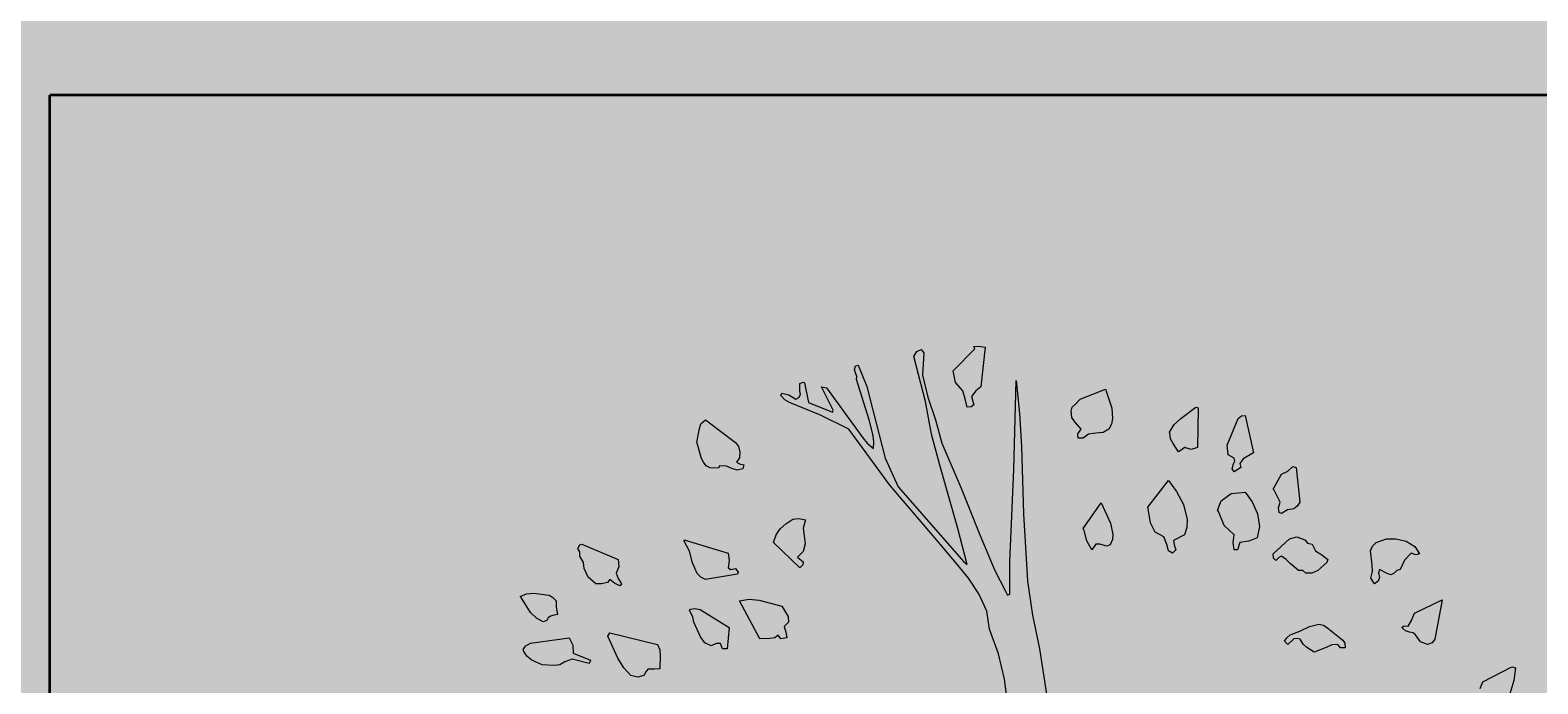
# Model space of a CAD drawing. Units: inches. Extents: x 84 to 1044, y -280 to 906.
# Tile 77 of 105: x 704 to 733, y 500 to 512. Entities that reach past the tile are written whole.
import ezdxf

# ---------------------------------------------------------------- set-up
doc = ezdxf.new("R2010")
doc.units = ezdxf.units.IN
for name, color, linetype, lineweight in [('A-ANNO-DIMS', 2, 'Continuous', 18), ('L-PLNT', 114, 'Continuous', 15), ('WALL', 250, 'Continuous', 35)]:
    doc.layers.add(name, color=color, linetype=linetype, lineweight=lineweight)
doc.layers.add('A-WALL-PATT', color=251, linetype='Continuous', lineweight=9, true_color=0x636466)
doc.layers.add('L-PLNT-PATT', color=9, linetype='Continuous', lineweight=9, true_color=0xafd9aa)
doc.styles.get("Standard").update_dxf_attribs({"font": 'arial.ttf'})
doc.dimstyles.get("Standard").update_dxf_attribs({"dimtxt": 0.18, "dimasz": 0.18, "dimexe": 0.18, "dimexo": 0.0625, "dimgap": 0.09, "dimtad": 0, "dimtih": 1, "dimtoh": 1, "dimdec": 4, "dimzin": 0, "dimdsep": 46, "dimtxsty": 'Standard', "dimcen": 0.09, "dimadec": 0, "dimazin": 0, "dimtfac": 1, "dimtdec": 4, "dimtofl": 0, "dimtmove": 0, "dimatfit": 3, "dimfxl": 1, "dimtolj": 1, "dimtzin": 0, "dimarcsym": 0})

# ---------------------------------------------------------------- blocks, each defined once
blk = doc.blocks.new('A$C37E508DF')
for p, q in [((0.6329, 1.5111), (0.6367, 1.5175)), ((0.6367, 1.5175), (0.6423, 1.5201)), ((0.6423, 1.5201), (0.6453, 1.5158)), ((0.6826, 1.493), (0.7096, 1.5209)), ((0.7083, 1.5239), (0.7152, 1.5244)), ((0.7096, 1.5209), (0.7083, 1.5239)), ((0.7152, 1.5244), (0.7225, 1.5231)), ((0.7225, 1.5231), (0.7174, 1.4729)), ((0.5583, 1.4948), (0.5596, 1.4995)), ((0.5596, 1.4995), (0.563, 1.5003)), ((0.563, 1.5003), (0.5737, 1.4733)), ((0.6475, 1.4545), (0.6329, 1.5111)), ((0.6453, 1.5158), (0.644, 1.4879)), ((0.5596, 1.4905), (0.5583, 1.4948)), ((0.5613, 1.4862), (0.5596, 1.4905)), ((0.5608, 1.4823), (0.5613, 1.4862)), ((0.5767, 1.4317), (0.5608, 1.4823)), ((0.644, 1.4879), (0.6505, 1.46)), ((0.6852, 1.4785), (0.6826, 1.493)), ((0.7589, 1.3691), (0.7615, 1.481)), ((0.7615, 1.481), (0.7658, 1.4395)), ((0.4657, 1.4622), (0.4669, 1.4652)), ((0.4708, 1.4566), (0.4657, 1.4622)), ((0.4669, 1.4652), (0.4755, 1.463)), ((0.4755, 1.463), (0.4845, 1.4575)), ((0.4884, 1.4596), (0.4905, 1.4635)), ((0.4897, 1.4772), (0.4935, 1.4789)), ((0.4897, 1.4678), (0.4897, 1.4772)), ((0.4905, 1.4635), (0.4897, 1.4678)), ((0.4935, 1.4789), (0.4952, 1.478)), ((0.4952, 1.478), (0.5004, 1.4532)), ((0.5313, 1.4437), (0.5167, 1.4729)), ((0.5167, 1.4729), (0.5231, 1.4716)), ((0.5231, 1.4716), (0.5686, 1.409)), ((0.5737, 1.4733), (0.5814, 1.4437)), ((0.6946, 1.4682), (0.6852, 1.4785)), ((0.6976, 1.4579), (0.6946, 1.4682)), ((0.7109, 1.4682), (0.7053, 1.4609)), ((0.7053, 1.4609), (0.7083, 1.4502)), ((0.7174, 1.4729), (0.7109, 1.4682)), ((0.8421, 1.4575), (0.8739, 1.4703)), ((0.8739, 1.4703), (0.882, 1.4463)), ((0.4764, 1.4532), (0.4708, 1.4566)), ((0.5154, 1.4373), (0.4764, 1.4532)), ((0.4845, 1.4575), (0.4884, 1.4596)), ((0.5004, 1.4532), (0.5308, 1.4412)), ((0.5308, 1.4412), (0.5313, 1.4437)), ((0.5814, 1.4437), (0.5969, 1.3833)), ((0.6552, 1.4137), (0.6475, 1.4545)), ((0.6505, 1.46), (0.6603, 1.4317)), ((0.7002, 1.4476), (0.6976, 1.4579)), ((0.7049, 1.448), (0.7002, 1.4476)), ((0.7083, 1.4502), (0.7049, 1.448)), ((0.831, 1.4424), (0.8323, 1.4476)), ((0.8318, 1.4343), (0.831, 1.4424)), ((0.8323, 1.4476), (0.8357, 1.451)), ((0.8357, 1.451), (0.8421, 1.4575)), ((0.882, 1.4463), (0.8829, 1.433)), ((0.9686, 1.4334), (0.9875, 1.4476)), ((0.9875, 1.4476), (0.9905, 1.4467)), ((0.9905, 1.4467), (0.9896, 1.3966)), ((0.3628, 1.4189), (0.3649, 1.4266)), ((0.3649, 1.4266), (0.3709, 1.4317)), ((0.3709, 1.4317), (0.4086, 1.403)), ((0.551, 1.4197), (0.5154, 1.4373)), ((0.5814, 1.4133), (0.5767, 1.4317)), ((0.6603, 1.4317), (0.668, 1.4021)), ((0.7658, 1.4395), (0.7684, 1.3979)), ((0.8353, 1.4292), (0.8318, 1.4343)), ((0.8434, 1.4197), (0.8353, 1.4292)), ((0.8816, 1.4262), (0.8781, 1.4197)), ((0.8829, 1.433), (0.8816, 1.4262)), ((0.9545, 1.4159), (0.9605, 1.4257)), ((0.9605, 1.4257), (0.9686, 1.4334)), ((1.0269, 1.3996), (1.0411, 1.433)), ((1.0411, 1.433), (1.045, 1.4365)), ((1.045, 1.4365), (1.0497, 1.4369)), ((1.0497, 1.4369), (1.0604, 1.3901)), ((0.3598, 1.403), (0.3628, 1.4189)), ((0.6029, 1.3494), (0.551, 1.4197)), ((0.5686, 1.409), (0.5741, 1.4021)), ((0.5827, 1.4043), (0.5814, 1.4133)), ((0.5823, 1.3953), (0.5827, 1.4043)), ((0.6655, 1.3743), (0.6552, 1.4137)), ((0.8391, 1.4141), (0.8434, 1.4197)), ((0.8395, 1.4086), (0.8391, 1.4141)), ((0.846, 1.4086), (0.8395, 1.4086)), ((0.8528, 1.4137), (0.846, 1.4086)), ((0.8619, 1.4146), (0.8528, 1.4137)), ((0.8709, 1.4154), (0.8619, 1.4146)), ((0.8781, 1.4197), (0.8709, 1.4154)), ((0.9549, 1.4146), (0.9545, 1.4159)), ((0.9558, 1.4077), (0.9549, 1.4146)), ((0.9592, 1.4017), (0.9558, 1.4077)), ((0.3602, 1.4021), (0.3598, 1.403)), ((0.364, 1.3888), (0.3602, 1.4021)), ((0.3657, 1.3828), (0.364, 1.3888)), ((0.4086, 1.403), (0.4125, 1.3979)), ((0.4125, 1.3979), (0.4142, 1.391)), ((0.4142, 1.391), (0.4134, 1.3837)), ((0.5741, 1.4021), (0.5823, 1.3953)), ((0.668, 1.4021), (0.6925, 1.3455)), ((0.7684, 1.3979), (0.771, 1.3134)), ((0.966, 1.3914), (0.9592, 1.4017)), ((0.9703, 1.3944), (0.966, 1.3914)), ((0.9733, 1.3966), (0.9703, 1.3944)), ((0.9819, 1.3944), (0.9733, 1.3966)), ((0.9896, 1.3966), (0.9819, 1.3944)), ((1.0282, 1.3876), (1.0269, 1.3996)), ((1.0359, 1.3833), (1.0282, 1.3876)), ((1.0604, 1.3901), (1.0471, 1.3824)), ((0.3683, 1.3781), (0.3657, 1.3828)), ((0.3718, 1.3738), (0.3683, 1.3781)), ((0.3765, 1.3713), (0.3718, 1.3738)), ((0.3872, 1.3708), (0.3765, 1.3713)), ((0.3885, 1.3738), (0.3872, 1.3708)), ((0.3971, 1.3734), (0.3885, 1.3738)), ((0.4039, 1.3704), (0.3971, 1.3734)), ((0.4108, 1.3683), (0.4039, 1.3704)), ((0.4134, 1.3837), (0.4099, 1.3781)), ((0.4099, 1.3781), (0.4134, 1.376)), ((0.4176, 1.37), (0.4108, 1.3683)), ((0.4134, 1.376), (0.4189, 1.3751)), ((0.4189, 1.3751), (0.4176, 1.37)), ((0.5969, 1.3833), (0.6132, 1.3472)), ((0.6882, 1.2949), (0.6655, 1.3743)), ((0.7538, 1.2529), (0.7589, 1.3691)), ((1.0334, 1.37), (1.0351, 1.376)), ((1.0359, 1.3661), (1.0334, 1.37)), ((1.0351, 1.376), (1.0368, 1.3794)), ((1.0368, 1.3794), (1.0359, 1.3833)), ((1.0441, 1.3717), (1.0359, 1.3661)), ((1.0471, 1.3824), (1.0432, 1.3764)), ((1.0432, 1.3764), (1.0441, 1.3717)), ((1.0955, 1.3631), (1.1033, 1.367)), ((1.1033, 1.367), (1.1097, 1.373)), ((1.1097, 1.373), (1.114, 1.3717)), ((1.114, 1.3717), (1.1183, 1.328)), ((0.6595, 1.2829), (0.6029, 1.3494)), ((0.6132, 1.3472), (0.6959, 1.2529)), ((0.9274, 1.3215), (0.9532, 1.3554)), ((0.9532, 1.3554), (0.9635, 1.3413)), ((1.0848, 1.3443), (1.0955, 1.3631)), ((0.6925, 1.3455), (0.7161, 1.2868)), ((0.9635, 1.3413), (0.9721, 1.325)), ((1.0171, 1.3232), (1.0197, 1.3297)), ((1.0197, 1.3297), (1.0321, 1.3387)), ((1.0321, 1.3387), (1.0497, 1.3404)), ((1.0497, 1.3404), (1.0587, 1.3284)), ((1.0587, 1.3284), (1.0651, 1.3134)), ((1.0861, 1.343), (1.0848, 1.3443)), ((1.0938, 1.328), (1.0861, 1.343)), ((1.0917, 1.3207), (1.0938, 1.328)), ((1.1183, 1.328), (1.1153, 1.3228)), ((0.771, 1.3134), (0.7761, 1.2285)), ((0.846, 1.2949), (0.8687, 1.3271)), ((0.8687, 1.3271), (0.8803, 1.3014)), ((0.9279, 1.3194), (0.9274, 1.3215)), ((0.9305, 1.3018), (0.9279, 1.3194)), ((0.9721, 1.325), (0.9768, 1.3061)), ((1.0149, 1.3172), (1.0171, 1.3232)), ((1.0162, 1.3164), (1.0149, 1.3172)), ((1.0231, 1.2988), (1.0162, 1.3164)), ((1.0651, 1.3134), (1.0677, 1.2975)), ((1.0925, 1.3151), (1.0917, 1.3207)), ((1.0955, 1.3138), (1.0925, 1.3151)), ((1.1028, 1.3185), (1.0955, 1.3138)), ((1.111, 1.3194), (1.1028, 1.3185)), ((1.1153, 1.3228), (1.111, 1.3194)), ((0.4597, 1.2868), (0.4648, 1.2945)), ((0.4648, 1.2945), (0.4717, 1.3009)), ((0.4717, 1.3009), (0.4807, 1.3065)), ((0.4807, 1.3065), (0.4884, 1.3074)), ((0.4884, 1.3074), (0.4965, 1.3057)), ((0.4965, 1.3057), (0.4935, 1.2954)), ((0.4935, 1.2954), (0.4948, 1.2855)), ((0.7002, 1.2495), (0.6882, 1.2949)), ((0.8473, 1.2924), (0.846, 1.2949)), ((0.8507, 1.2795), (0.8473, 1.2924)), ((0.8803, 1.3014), (0.8833, 1.2872)), ((0.9365, 1.2902), (0.9305, 1.3018)), ((0.9476, 1.2842), (0.9365, 1.2902)), ((0.9763, 1.2962), (0.9733, 1.2868)), ((0.9768, 1.3061), (0.9763, 1.2962)), ((1.0359, 1.2868), (1.0231, 1.2988)), ((1.0677, 1.2975), (1.0647, 1.2829)), ((0.2101, 1.2696), (0.2127, 1.2744)), ((0.2127, 1.2744), (0.2152, 1.2752)), ((0.2152, 1.2752), (0.2611, 1.2559)), ((0.3439, 1.2804), (0.3992, 1.2636)), ((0.3439, 1.2787), (0.3439, 1.2804)), ((0.3507, 1.2662), (0.3439, 1.2787)), ((0.4562, 1.2774), (0.4597, 1.2868)), ((0.4897, 1.2452), (0.4562, 1.2774)), ((0.4961, 1.2756), (0.4935, 1.2658)), ((0.4948, 1.2855), (0.4961, 1.2756)), ((0.6865, 1.2508), (0.6595, 1.2829)), ((0.7161, 1.2868), (0.7349, 1.2422)), ((0.8567, 1.2679), (0.8507, 1.2795)), ((0.8619, 1.2752), (0.8567, 1.2679)), ((0.867, 1.2752), (0.8619, 1.2752)), ((0.8713, 1.2739), (0.867, 1.2752)), ((0.8756, 1.2726), (0.8713, 1.2739)), ((0.8799, 1.2744), (0.8756, 1.2726)), ((0.8829, 1.2808), (0.8799, 1.2744)), ((0.8833, 1.2872), (0.8829, 1.2808)), ((0.951, 1.2748), (0.9476, 1.2842)), ((0.9532, 1.2666), (0.951, 1.2748)), ((0.9733, 1.2868), (0.9596, 1.2799)), ((0.9596, 1.2799), (0.9605, 1.2744)), ((0.9605, 1.2744), (0.9626, 1.2679)), ((1.0347, 1.2769), (1.0359, 1.2868)), ((1.0359, 1.2679), (1.0347, 1.2769)), ((1.0432, 1.2774), (1.0402, 1.2679)), ((1.0544, 1.2791), (1.0432, 1.2774)), ((1.0647, 1.2829), (1.0544, 1.2791)), ((1.0848, 1.2628), (1.1054, 1.2817)), ((1.1054, 1.2817), (1.1148, 1.2842)), ((1.1148, 1.2842), (1.1247, 1.2804)), ((1.1247, 1.2804), (1.1281, 1.2765)), ((1.1281, 1.2765), (1.1341, 1.2752)), ((1.1341, 1.2752), (1.1384, 1.2666)), ((1.2075, 1.2666), (1.21, 1.2726)), ((1.21, 1.2726), (1.2147, 1.2774)), ((1.2147, 1.2774), (1.2276, 1.2817)), ((1.2276, 1.2817), (1.2392, 1.2817)), ((1.2392, 1.2817), (1.2521, 1.2787)), ((1.2521, 1.2787), (1.2632, 1.2722)), ((1.2632, 1.2722), (1.2692, 1.2628)), ((0.2127, 1.2654), (0.2101, 1.2696)), ((0.2127, 1.2602), (0.2127, 1.2654)), ((0.2174, 1.2521), (0.2127, 1.2602)), ((0.2182, 1.2443), (0.2174, 1.2521)), ((0.2611, 1.2559), (0.262, 1.2465)), ((0.3546, 1.2516), (0.3507, 1.2662)), ((0.3992, 1.2636), (0.4005, 1.2546)), ((0.4005, 1.2546), (0.3992, 1.2452)), ((0.4935, 1.2658), (0.4867, 1.2589)), ((0.4867, 1.2589), (0.4935, 1.2529)), ((0.4935, 1.2529), (0.4931, 1.2491)), ((0.6959, 1.2529), (0.7002, 1.2495)), ((0.7538, 1.2122), (0.7538, 1.2529)), ((0.9583, 1.2636), (0.9532, 1.2666)), ((0.9626, 1.2679), (0.9583, 1.2636)), ((1.0402, 1.2679), (1.0359, 1.2679)), ((1.0852, 1.2576), (1.0848, 1.2628)), ((1.0883, 1.2546), (1.0852, 1.2576)), ((1.0921, 1.2585), (1.0883, 1.2546)), ((1.0955, 1.2602), (1.0921, 1.2585)), ((1.1015, 1.2559), (1.0955, 1.2602)), ((1.1063, 1.2508), (1.1015, 1.2559)), ((1.1384, 1.2666), (1.1461, 1.2619)), ((1.1526, 1.2521), (1.141, 1.2422)), ((1.1461, 1.2619), (1.1539, 1.2559)), ((1.1539, 1.2559), (1.1526, 1.2521)), ((1.2096, 1.2491), (1.2075, 1.2666)), ((1.2503, 1.2551), (1.2448, 1.2431)), ((1.2585, 1.2636), (1.2503, 1.2551)), ((1.2645, 1.2615), (1.2585, 1.2636)), ((1.2692, 1.2628), (1.2645, 1.2615)), ((0.2234, 1.2336), (0.2182, 1.2443)), ((0.2328, 1.2251), (0.2234, 1.2336)), ((0.262, 1.2465), (0.2586, 1.2388)), ((0.2586, 1.2388), (0.2611, 1.2319)), ((0.3602, 1.2383), (0.3546, 1.2516)), ((0.3649, 1.2336), (0.3602, 1.2383)), ((0.3709, 1.2306), (0.3649, 1.2336)), ((0.4112, 1.2375), (0.3709, 1.2306)), ((0.3992, 1.2452), (0.4026, 1.2431)), ((0.4026, 1.2431), (0.4086, 1.2443)), ((0.4086, 1.2443), (0.4121, 1.2401)), ((0.4121, 1.2401), (0.4112, 1.2375)), ((0.4931, 1.2491), (0.4897, 1.2452)), ((0.7015, 1.2323), (0.6865, 1.2508)), ((0.7349, 1.2422), (0.7482, 1.216)), ((1.117, 1.2422), (1.1063, 1.2508)), ((1.1221, 1.2418), (1.117, 1.2422)), ((1.126, 1.2388), (1.1221, 1.2418)), ((1.1337, 1.2388), (1.126, 1.2388)), ((1.141, 1.2422), (1.1337, 1.2388)), ((1.2079, 1.2323), (1.21, 1.2409)), ((1.21, 1.2409), (1.2096, 1.2491)), ((1.2186, 1.2332), (1.2169, 1.2285)), ((1.2186, 1.2431), (1.2173, 1.2392)), ((1.2173, 1.2392), (1.2186, 1.2332)), ((1.2285, 1.2383), (1.2186, 1.2431)), ((1.2328, 1.2366), (1.2285, 1.2383)), ((1.2371, 1.2388), (1.2328, 1.2366)), ((1.2405, 1.2418), (1.2371, 1.2388)), ((1.2448, 1.2431), (1.2405, 1.2418)), ((0.2401, 1.2251), (0.2328, 1.2251)), ((0.2474, 1.2268), (0.2401, 1.2251)), ((0.2504, 1.2306), (0.2474, 1.2268)), ((0.2568, 1.2255), (0.2504, 1.2306)), ((0.2633, 1.2229), (0.2568, 1.2255)), ((0.2611, 1.2319), (0.265, 1.2251)), ((0.265, 1.2251), (0.2633, 1.2229)), ((0.7148, 1.2126), (0.7015, 1.2323)), ((0.7482, 1.216), (0.7508, 1.2109)), ((0.7761, 1.2285), (0.7821, 1.1856)), ((1.2126, 1.2251), (1.2079, 1.2323)), ((1.2169, 1.2285), (1.2126, 1.2251)), ((0.1376, 1.2092), (0.1458, 1.2126)), ((0.1389, 1.2079), (0.1376, 1.2092)), ((0.1505, 1.189), (0.1389, 1.2079)), ((0.1458, 1.2126), (0.1548, 1.2135)), ((0.1548, 1.2135), (0.1741, 1.2109)), ((0.1741, 1.2109), (0.1784, 1.2083)), ((0.1784, 1.2083), (0.1831, 1.204)), ((0.1831, 1.204), (0.1831, 1.1959)), ((0.1831, 1.1959), (0.1848, 1.1865)), ((0.4134, 1.204), (0.4258, 1.2058)), ((0.4391, 1.156), (0.4134, 1.204)), ((0.4258, 1.2058), (0.4382, 1.2045)), ((0.4382, 1.2045), (0.4669, 1.1972)), ((0.4669, 1.1972), (0.4747, 1.1843)), ((0.7246, 1.1908), (0.7148, 1.2126)), ((0.7508, 1.2109), (0.7538, 1.2122)), ((1.2628, 1.1882), (1.2975, 1.2053)), ((1.2975, 1.2053), (1.2885, 1.1556)), ((0.1582, 1.1822), (0.1505, 1.189)), ((0.1668, 1.1775), (0.1582, 1.1822)), ((0.1711, 1.1792), (0.1668, 1.1775)), ((0.1728, 1.1826), (0.1711, 1.1792)), ((0.1758, 1.1847), (0.1728, 1.1826)), ((0.1788, 1.1852), (0.1758, 1.1847)), ((0.1848, 1.1865), (0.1788, 1.1852)), ((0.3507, 1.1916), (0.352, 1.1933)), ((0.355, 1.1839), (0.3507, 1.1916)), ((0.352, 1.1933), (0.3576, 1.1942)), ((0.3563, 1.177), (0.355, 1.1839)), ((0.3645, 1.1586), (0.3563, 1.177)), ((0.3576, 1.1942), (0.364, 1.1929)), ((0.364, 1.1929), (0.4005, 1.1702)), ((0.4751, 1.177), (0.47, 1.1714)), ((0.4747, 1.1843), (0.4751, 1.177)), ((0.7281, 1.168), (0.7246, 1.1908)), ((0.7821, 1.1856), (0.7911, 1.1436)), ((1.2546, 1.1719), (1.2589, 1.1792)), ((1.2589, 1.1792), (1.2628, 1.1882)), ((0.1509, 1.1504), (0.1994, 1.1573)), ((0.1994, 1.1573), (0.2041, 1.1479)), ((0.2478, 1.1594), (0.2504, 1.1637)), ((0.2607, 1.1316), (0.2478, 1.1594)), ((0.2504, 1.1637), (0.3104, 1.1487)), ((0.37, 1.1509), (0.3645, 1.1586)), ((0.4005, 1.1702), (0.3979, 1.1436)), ((0.458, 1.1573), (0.4519, 1.1564)), ((0.4622, 1.1607), (0.458, 1.1573)), ((0.4657, 1.156), (0.4622, 1.1607)), ((0.473, 1.1573), (0.4657, 1.156)), ((0.47, 1.1714), (0.4721, 1.1646)), ((0.4721, 1.1646), (0.473, 1.1573)), ((0.7396, 1.1371), (0.7281, 1.168)), ((1.099, 1.153), (1.102, 1.1573)), ((1.102, 1.1573), (1.1063, 1.1612)), ((1.1063, 1.1612), (1.1187, 1.1655)), ((1.1187, 1.1655), (1.1307, 1.1714)), ((1.1307, 1.1714), (1.1423, 1.1744)), ((1.1423, 1.1744), (1.1483, 1.1732)), ((1.1483, 1.1732), (1.1539, 1.1693)), ((1.1539, 1.1693), (1.1727, 1.1543)), ((1.2469, 1.1702), (1.2495, 1.1723)), ((1.2478, 1.1693), (1.2469, 1.1702)), ((1.2516, 1.1659), (1.2478, 1.1693)), ((1.2495, 1.1723), (1.2546, 1.1719)), ((1.2563, 1.1646), (1.2516, 1.1659)), ((1.2611, 1.1637), (1.2563, 1.1646)), ((1.2641, 1.1612), (1.2611, 1.1637)), ((1.2701, 1.1522), (1.2641, 1.1612)), ((0.1419, 1.1436), (0.1449, 1.1474)), ((0.1419, 1.141), (0.1419, 1.1436)), ((0.1462, 1.1342), (0.1419, 1.141)), ((0.1449, 1.1474), (0.1509, 1.1504)), ((0.2041, 1.1479), (0.2045, 1.138)), ((0.2045, 1.138), (0.226, 1.129)), ((0.3104, 1.1487), (0.3134, 1.1423)), ((0.3134, 1.1423), (0.3139, 1.1346)), ((0.3778, 1.1474), (0.37, 1.1509)), ((0.3842, 1.15), (0.3778, 1.1474)), ((0.3898, 1.15), (0.3842, 1.15)), ((0.3923, 1.1436), (0.3898, 1.15)), ((0.3979, 1.1436), (0.3923, 1.1436)), ((0.4519, 1.1564), (0.4391, 1.156)), ((0.7911, 1.1436), (0.8027, 1.0677)), ((1.1033, 1.1487), (1.099, 1.153)), ((1.111, 1.156), (1.1033, 1.1487)), ((1.1153, 1.1564), (1.111, 1.156)), ((1.1191, 1.1556), (1.1153, 1.1564)), ((1.1226, 1.1492), (1.1191, 1.1556)), ((1.1273, 1.1453), (1.1226, 1.1492)), ((1.1367, 1.1393), (1.1273, 1.1453)), ((1.1517, 1.1453), (1.1367, 1.1393)), ((1.1586, 1.1483), (1.1517, 1.1453)), ((1.1663, 1.1487), (1.1586, 1.1483)), ((1.1697, 1.1449), (1.1663, 1.1487)), ((1.1757, 1.1449), (1.1697, 1.1449)), ((1.1727, 1.1543), (1.1749, 1.1504)), ((1.1749, 1.1504), (1.1757, 1.1449)), ((1.2791, 1.1487), (1.2701, 1.1522)), ((1.2851, 1.1509), (1.2791, 1.1487)), ((1.2885, 1.1556), (1.2851, 1.1509)), ((0.1522, 1.1294), (0.1462, 1.1342)), ((0.1655, 1.1234), (0.1522, 1.1294)), ((0.181, 1.1226), (0.1655, 1.1234)), ((0.1878, 1.1234), (0.181, 1.1226)), ((0.1938, 1.1273), (0.1878, 1.1234)), ((0.2032, 1.1303), (0.1938, 1.1273)), ((0.2247, 1.1251), (0.2032, 1.1303)), ((0.226, 1.129), (0.2247, 1.1251)), ((0.268, 1.1196), (0.2607, 1.1316)), ((0.277, 1.1101), (0.268, 1.1196)), ((0.3139, 1.1346), (0.3134, 1.1183)), ((0.7469, 1.1054), (0.7396, 1.1371)), ((1.3485, 1.102), (1.385, 1.1209)), ((1.385, 1.1209), (1.3897, 1.1196)), ((1.3897, 1.1196), (1.3875, 1.1037)), ((0.2856, 1.108), (0.277, 1.1101)), ((0.2933, 1.1101), (0.2856, 1.108)), ((0.2959, 1.1144), (0.2933, 1.1101)), ((0.2984, 1.1179), (0.2959, 1.1144)), ((0.3066, 1.1179), (0.2984, 1.1179)), ((0.3134, 1.1183), (0.3066, 1.1179)), ((0.7512, 1.0728), (0.7469, 1.1054)), ((1.3455, 1.0934), (1.3485, 1.102)), ((1.3875, 1.1037), (1.3828, 1.087))]:
    blk.add_line(p, q)
blk = doc.blocks.new('*D62')
at = {"layer": 'A-ANNO-DIMS', "color": 0, "lineweight": -2, "transparency": 16777216}
for p, q in [((203.179, 709.183), (203.179, 905.9)), ((896.074, 400.183), (896.074, 905.9)), ((203.359, 905.72), (549.232, 905.72)), ((895.894, 905.72), (550.021, 905.72))]:
    blk.add_line(p, q, dxfattribs=at)
at = {"layer": 'A-ANNO-DIMS', "color": 0, "transparency": 16777216}
for points in [[(203.359, 905.75), (203.359, 905.69), (203.179, 905.72)], [(895.894, 905.75), (895.894, 905.69), (896.074, 905.72)]]:
    blk.add_solid(points, dxfattribs=at)
at = {"layer": 'Defpoints', "color": 0, "transparency": 16777216}
for p in [(896.074, 905.72), (203.179, 709.12), (896.074, 400.12)]:
    blk.add_point(p, dxfattribs=at)
at = {"layer": 'A-ANNO-DIMS', "color": 0, "transparency": 16777216, "insert": (549.627, 905.72), "char_height": 0.18, "attachment_point": 5}
blk.add_mtext('\\A1;692.9', dxfattribs=at)

msp = doc.modelspace()

# ---------------------------------------------------------------- hatches: boundary and pattern name
at = {"layer": 'A-WALL-PATT', "transparency": 33554597}
h = msp.add_hatch(color=256, dxfattribs=at)
h.dxf.hatch_style = 1
h.paths.add_polyline_path([(671.074, 100.12), (647.074, 100.12), (647.074, 160.12), (641.074, 160.12), (620.824, 160.12), (620.824, 151.12), (638.074, 151.12), (638.074, 91.12), (671.074, 91.12)])
h.paths.add_polyline_path([(791.074, 100.12), (743.074, 100.12), (743.074, 91.12), (791.074, 91.12)])
h.paths.add_polyline_path([(896.074, 346.12), (887.074, 346.12), (887.074, 334.12), (870.955, 334.12), (833.074, 334.12), (804.574, 334.12), (804.574, 328.12), (887.074, 328.12), (887.074, 100.12), (863.074, 100.12), (863.074, 91.12), (896.074, 91.12)])
h.paths.add_polyline_path([(507.574, 154.729), (507.574, 160.12), (464.074, 160.12), (464.074, 247.12), (641.074, 247.12), (641.074, 208.12), (647.074, 208.12), (647.074, 328.12), (659.074, 328.12), (659.074, 334.12), (617.074, 334.12), (617.074, 328.12), (641.074, 328.12), (641.074, 256.12), (545.074, 256.12), (545.074, 328.12), (569.074, 328.12), (569.074, 334.12), (518.074, 334.12), (518.074, 325.12), (536.074, 325.12), (536.074, 256.12), (464.074, 256.12), (464.074, 325.12), (482.074, 325.12), (482.074, 334.12), (455.074, 334.12), (455.074, 160.12), (413.127, 160.12), (413.127, 151.12), (455.074, 151.12), (455.074, 91.12), (464.074, 91.12), (464.074, 151.12), (507.574, 151.12)])
h.paths.add_polyline_path([(572.824, 160.12), (555.574, 160.12), (555.574, 151.12), (572.824, 151.12)], flags=17)
h.paths.add_polyline_path([(341.127, 160.12), (299.179, 160.12), (299.179, 211.12), (294.179, 211.12), (290.179, 211.12), (290.179, 151.12), (341.127, 151.12)])
h.paths.add_polyline_path([(299.179, 256.12), (212.179, 256.12), (212.179, 274.12), (203.179, 274.12), (203.179, 247.12), (299.179, 247.12)])
h.paths.add_polyline_path([(212.179, 514.12), (398.074, 514.12), (398.074, 519.12), (398.074, 520.12), (212.179, 520.12), (212.179, 574.12), (203.179, 574.12), (203.179, 310.12), (212.179, 310.12), (212.179, 328.12), (290.179, 328.12), (290.179, 292.12), (299.179, 292.12), (299.179, 328.12), (332.179, 328.12), (332.179, 334.12), (212.179, 334.12)])
h.paths.add_polyline_path([(287.127, 709.12), (203.179, 709.12), (203.179, 646.12), (212.179, 646.12), (212.179, 700.12), (287.127, 700.12)])
h.paths.add_polyline_path([(470.074, 709.12), (359.127, 709.12), (359.127, 700.12), (434.074, 700.12), (434.074, 574.12), (440.074, 574.12), (440.074, 622.12), (464.074, 622.12), (464.074, 628.12), (440.074, 628.12), (440.074, 700.12), (470.074, 700.12)])
h.paths.add_polyline_path([(572.074, 709.12), (506.074, 709.12), (506.074, 700.12), (536.074, 700.12), (536.074, 628.12), (494.074, 628.12), (494.074, 622.12), (536.074, 622.12), (536.074, 520.12), (440.074, 520.12), (440.074, 544.12), (434.074, 544.12), (434.074, 514.12), (644.074, 514.12), (644.074, 519.12), (644.074, 544.12), (638.074, 544.12), (638.074, 520.12), (542.074, 520.12), (542.074, 622.12), (584.074, 622.12), (584.074, 628.12), (542.074, 628.12), (542.074, 700.12), (572.074, 700.12)])
h.paths.add_polyline_path([(698.074, 709.12), (608.074, 709.12), (608.074, 700.12), (638.074, 700.12), (638.074, 628.12), (614.074, 628.12), (614.074, 622.12), (638.074, 622.12), (638.074, 574.12), (644.074, 574.12), (644.074, 700.12), (698.074, 700.12)])
h.paths.add_polyline_path([(833.074, 709.12), (770.074, 709.12), (770.074, 700.12), (824.074, 700.12), (824.074, 646.12), (833.074, 646.12)])
h.paths.add_polyline_path([(833.074, 574.12), (824.074, 574.12), (824.074, 520.12), (791.244, 520.12), (712.904, 520.12), (680.074, 520.12), (680.074, 514.12), (695.074, 514.12), (695.074, 491.62), (704.074, 491.62), (704.074, 511.12), (833.074, 511.12)])
h.paths.add_polyline_path([(704.074, 419.62), (695.074, 419.62), (695.074, 370.12), (704.074, 370.12)])
h.paths.add_polyline_path([(896.074, 400.12), (833.074, 400.12), (833.074, 364.12), (839.074, 364.12), (839.074, 394.12), (887.074, 394.12), (887.074, 382.12), (896.074, 382.12)])
h.paths.add_polyline_path([(732.574, 334.12), (695.074, 334.12), (695.074, 328.12), (732.574, 328.12)])
at = {"layer": 'L-PLNT-PATT', "transparency": 33554597}
h = msp.add_hatch(color=256, dxfattribs=at)
h.dxf.hatch_style = 1
h.paths.add_polyline_path([(896.074, 511.12), (704.074, 511.12), (704.074, 491.62), (704.074, 419.62), (704.074, 400.12), (833.074, 400.12), (896.074, 400.12)])

# ---------------------------------------------------------------- linework, layer by layer
at = {"layer": 'WALL'}
for p in [(896.074, 511.12), (704.074, 491.62)]:
    msp.add_line(p, (704.074, 511.12), dxfattribs=at)

# ---------------------------------------------------------------- block references
at = {"layer": 'L-PLNT', "xscale": 15.19586232982809, "yscale": 15.19586232982809, "zscale": 15.19586232982809}
msp.add_blockref('A$C37E508DF', (710.97, 483.159), dxfattribs=at)

# ---------------------------------------------------------------- dimensions: what is measured, and where the dimension line sits
at = {"layer": 'A-ANNO-DIMS'}
dim = msp.add_linear_dim(base=(896.074, 905.72), p1=(203.179, 709.12), p2=(896.074, 400.12), dimstyle='Standard', override={"dimdec": 1, "dimlfac": 1, "dimrnd": 0, "dimzin": 0, "dimdsep": 46, "dimlunit": 2}, dxfattribs=at)
dim.commit()
dim.dimension.update_dxf_attribs({"geometry": '*D62', "text_midpoint": (549.627, 905.72)})

doc.saveas('drawing.dxf')
